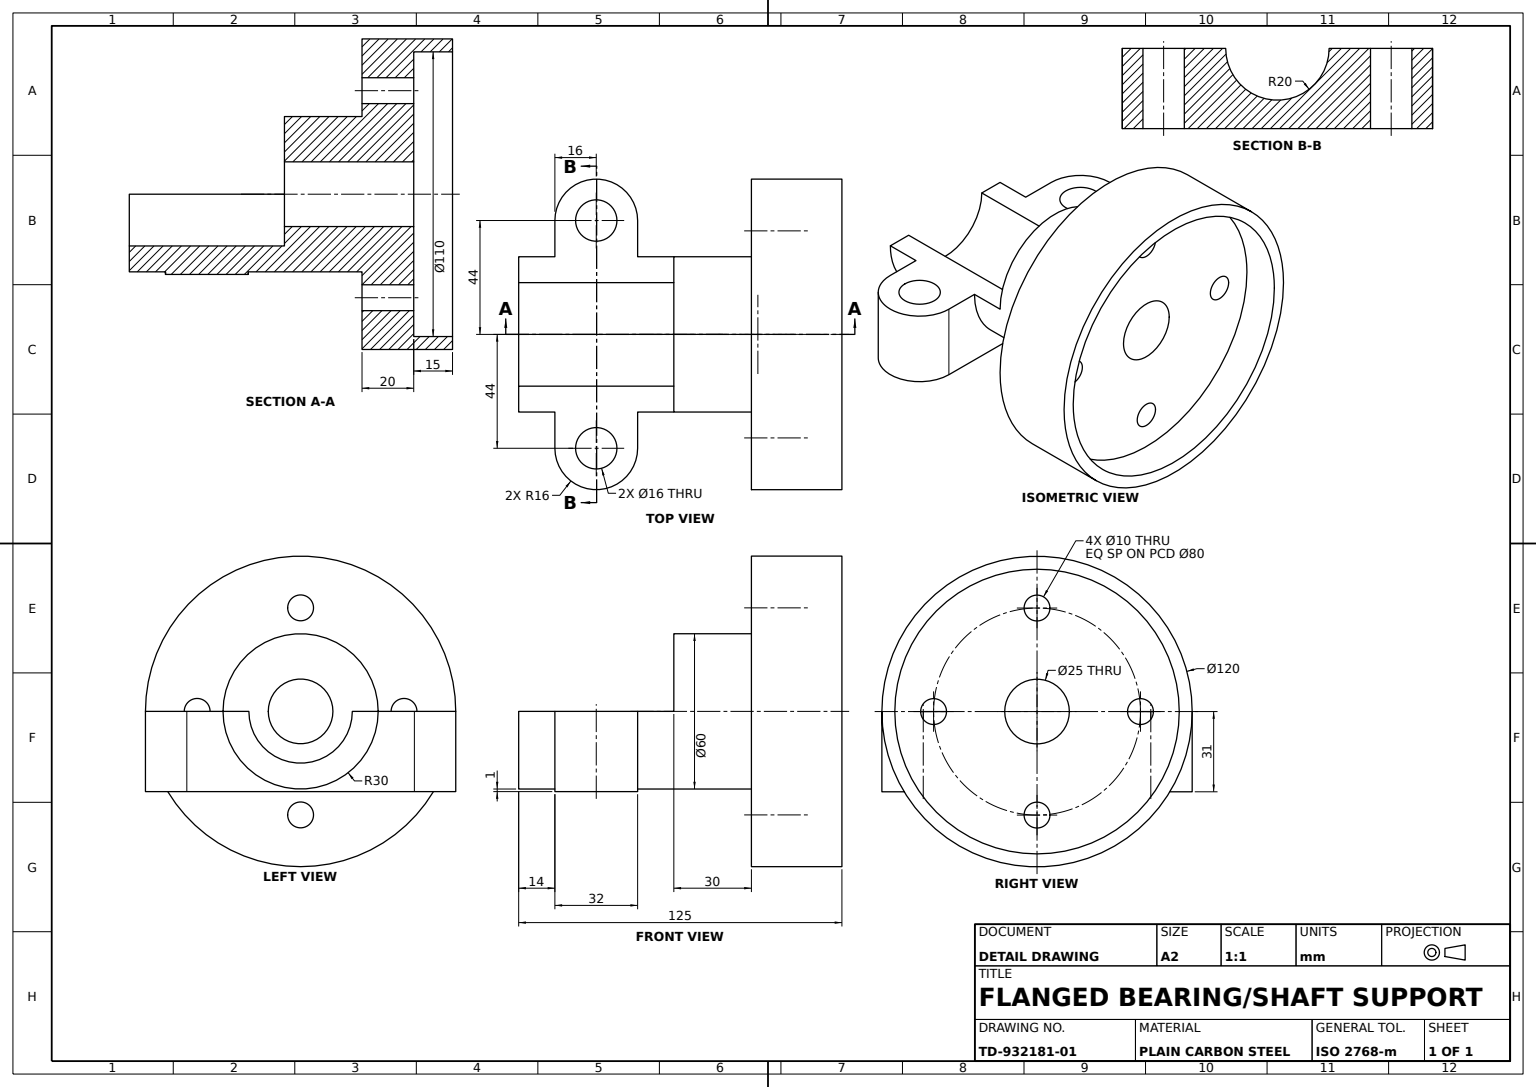
SolidWorks part; units mm, degrees
material "Plain Carbon Steel"
ref_plane "Front Plane" through (0, 0, 0) normal (0, 0, 1) x (1, 0, 0)
ref_plane "Top Plane" through (0, 0, 0) normal (0, 1, 0) x (1, 0, 0)
ref_plane "Right Plane" through (0, 0, 0) normal (1, 0, 0) x (0, 0, -1)
sketch "Base Flange Sketch" plane through (0, 0, 0) normal (0, 0, 1) x (1, 0, 0)
  circle A0 centre (0, 0) radius 55
  circle A1 centre (0, 0) radius 60
  dimension "D1" = 120
  dimension "D2" = 110
extrude "Base Flange Plate" add sketch "Base Flange Sketch" along normal blind 15
sketch "Round Flange Sketch Ø120" plane through (0, 0, 15) normal (0, 0, 1) x (1, 0, 0)
  circle A0 centre (0, 0) radius 60
  dimension "D1" = 120
extrude "Round Flange Ø120" add sketch "Round Flange Sketch Ø120" along normal blind 20
sketch "Flange Bolt Holes Sketch" plane through (0, 0, 35) normal (0, 0, 1) x (1, 0, 0)
  circle A1 centre (0, 40) radius 5
  circle A2 centre (40, 0) radius 5
  circle A3 centre (0, -40) radius 5
  circle A4 centre (-40, 0) radius 5
  dimension "D1" = 40
  dimension "D2" = 10
  dimension "D4" = 40
  dimension "D5" = 40
  dimension "D6" = 40
  dimension "D3" = 4
extrude "Flange Bolt Holes 4xØ10" cut sketch "Flange Bolt Holes Sketch" against normal blind 20
sketch "Hub Boss Sketch" plane through (0, 0, 35) normal (0, 0, 1) x (1, 0, 0)
  circle A0 centre (0, 0) radius 30
  circle A1 centre (0, 0) radius 12.5
  dimension "D1" = 60
  dimension "D2" = 25
extrude "Hub Boss" add sketch "Hub Boss Sketch" along normal blind 30
sketch "Hub Bore Sketch Ø25" plane through (0, 0, 35) normal (0, 0, 1) x (1, 0, 0)
  circle A0 centre (0, 0) radius 12.5
  dimension "D1" = 25
extrude "Hub Bore Ø25" cut sketch "Hub Bore Sketch Ø25" against normal blind 30
sketch "Cradle Body Sketch" plane through (0, 0, 65) normal (0, 0, 1) x (1, 0, 0)
  line L0 (-30, 0) -> (-12.5, 0)
  line L1 (12.5, 0) -> (30, 0)
  arc A0 (-30, 0) -> (30, 0) centre (0, 0) ccw
  arc A1 (-12.5, 0) -> (12.5, 0) centre (0, 0) ccw
  dimension "D1" = 30
  dimension "D2" = 12.5
extrude "Cradle Body" add sketch "Cradle Body Sketch" along normal blind 60
sketch "Cradle Lugs Sketch" plane through (0, 0, 0) normal (0, 1, 0) x (1, 0, 0)
  line L0 (-12.5, -125) -> (-30, -125) construction
  line L1 (30, -125) -> (12.5, -125) construction
  line L2 (-44, -79) -> (-12.5, -79)
  line L3 (-12.5, -125) -> (-12.5, -65) construction
  line L4 (-12.5, -79) -> (12.5, -79)
  line L5 (-12.5, -111) -> (-44, -111)
  line L6 (44, -79) -> (12.5, -79)
  line L9 (-12.5, -111) -> (12.5, -111)
  line L10 (12.5, -125) -> (12.5, -65) construction
  line L11 (12.5, -111) -> (44, -111)
  circle A0 centre (-44, -95) radius 8
  circle A1 centre (-44, -95) radius 16
  circle A2 centre (44, -95) radius 8
  circle A3 centre (44, -95) radius 16
  line M5 (12.5, -65) -> (12.5, -125)
  line M7 (30, -125) -> (30, -65)
  dimension "D1" = 16
  dimension "D2" = 32
  dimension "D3" = 16
  dimension "D4" = 32
  dimension "D5" = 44
  dimension "D6" = 44
  dimension "D7" = 30
  dimension "D8" = 30
  dimension "D9" = 32
extrude "Cradle Mounting Lugs" add sketch "Cradle Lugs Sketch" against normal blind 31 separate body contours A1 A0 | A1 L5 L9 L4 L2 M5 | A3 L6 L11 M7 M5 | A3 L6 M7 | A3 L11 M7 | A3 A2 M7
sketch "Cradle Bore Sketch Ø40" plane through (0, 0, 125) normal (0, 0, 1) x (1, 0, 0)
  circle A0 centre (0, 0) radius 20
  dimension "D1" = 40
extrude "Cradle Bore Ø40" cut sketch "Cradle Bore Sketch Ø40" against normal blind 60
sketch "Lug Pad Sketch" plane through (0, -31, 0) normal (0, -1, 0) x (1, 0, 0)
  line L0 (-44, 111) -> (44, 111)
  line L1 (-44, 79) -> (44, 79)
  line L2 (30, 102.746) -> (30, 87.254) construction
  circle A0 centre (-44, 95) radius 16
  circle A1 centre (44, 95) radius 16
  circle A2 centre (44, 95) radius 8
  circle A3 centre (-44, 95) radius 8
  arc M3 (30, 87.254) -> (30, 102.746) centre (44, 95) cw
  line M4 (30, 102.746) -> (30, 87.254)
  circle M5 centre (-44, 95) radius 8
  arc M6 (-44, 111) -> (-44, 79) centre (-44, 95) ccw
  line M7 (-44, 79) -> (44, 79)
  arc M8 (44, 79) -> (44, 111) centre (44, 95) ccw
  line M9 (44, 111) -> (-44, 111)
  circle M10 centre (44, 95) radius 8
  dimension "D1" = 32
  dimension "D2" = 32
  dimension "D3" = 16
  dimension "D4" = 16
  dimension "D5" = 14
  dimension "D6" = 74
extrude "Lug Pads" add sketch "Lug Pad Sketch" against normal blind 32 contours A0 M6 M5 | A1 A0 M9 M7 M3 | M3 M4 | A1 M8 M4 M10
sketch "Parting Slot Sketch" plane through (0, 0, 111) normal (0, 0, 1) x (1, 0, 0)
  line L1 (-60, 1) -> (60, 1)
  line L2 (-60, 1) -> (-60, 0)
  line L3 (-60, 0) -> (60, 0)
  line L4 (60, 1) -> (60, 0)
  dimension "D1" = 1
  dimension "D2" = 120
extrude "Cradle Parting Slot 1mm" cut sketch "Parting Slot Sketch" against normal blind 32
sketch "Lug Bore Sketch Ø40" plane through (0, 0, 125) normal (0, 0, 1) x (1, 0, 0)
  circle A0 centre (0, 0) radius 20
  dimension "D1" = 40
extrude "Cradle Bore Ø40 Through Lugs" cut sketch "Lug Bore Sketch Ø40" against normal blind 60
